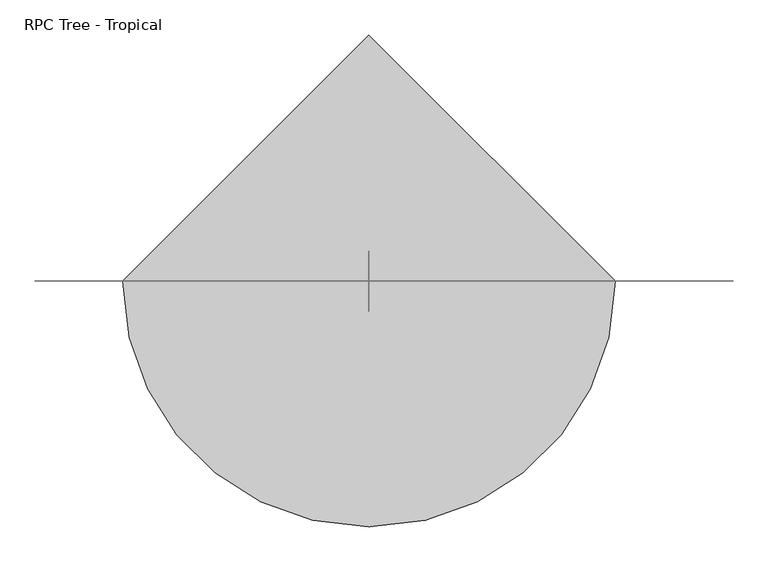
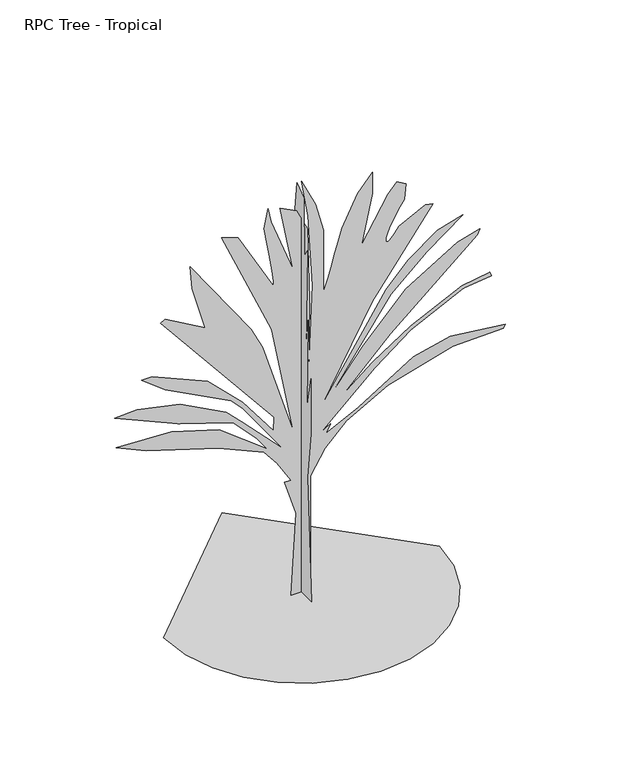
"""IFC4 building model written with IfcOpenShell, lengths in millimetres: geographic element geometry, RPC Tree - Tropical."""

from ifc_helpers import new_model, si_unit, origin, place, context, project, spatial, triangles, source, transform, mapped, element, save


def rpc_tree_tropical_0177ab4a(model_context):
    return source(origin(), model_context, "Body", "Tessellation", [
        triangles([(-93.7534889, -0.0079219, 0.0614497), (-47.9158571, -0.0079683, 779.2394274), (-154.8704887, -0.0079884, 1115.3806829), (-93.7534889, -0.0079881, 1110.2879705), (-221.0799467, -0.0080005, 1319.1040764), (-343.3142189, -0.0080096, 1471.8953316), (-755.8511021, -0.0080203, 1650.1526196), (-1417.9506592, -0.0080327, 1858.9686527), (-1692.9744244, -0.0080403, 1986.2938751), (-1183.6685932, -0.0080388, 1960.827697), (-750.7583897, -0.0080309, 1828.4099075), (-312.7554374, -0.0080109, 1492.2660358), (-409.5244217, -0.008019, 1629.7791538), (-623.4331673, -0.0080324, 1853.8733242), (-1122.5511028, -0.0080421, 2016.8526203), (-1708.2550323, -0.0080576, 2276.5982483), (-1499.4389992, -0.0080582, 2286.7861439), (-1107.2729656, -0.008053, 2200.2026207), (-689.6408993, -0.0080397, 1976.1084503), (-547.0350326, -0.0080312, 1833.5026199), (-170.149607, -0.0080081, 1446.4291534), (-531.7569317, -0.0080385, 1955.7349846), (-643.8040169, -0.0080455, 2072.8773983), (-1244.7860836, -0.0080643, 2388.6453335), (-1458.6948292, -0.0080743, 2556.7145805), (-1361.9258812, -0.0080743, 2556.7145805), (-857.7127625, -0.0080609, 2332.6230263), (-536.8496078, -0.0080424, 2021.9453327), (-256.7306412, -0.00802, 1645.0599072), (-251.6384557, -0.0080279, 1777.4776966), (-1285.5302536, -0.0081034, 3045.6393883), (-1244.7860836, -0.008105, 3071.1157402), (-878.0860828, -0.0080922, 2857.1968208), (-1000.3185928, -0.0081174, 3279.9291573), (-1015.5992735, -0.0081302, 3493.8480766), (-460.4539802, -0.0080828, 2699.3102371), (-353.4996074, -0.00807, 2485.4142815), (-73.3816582, -0.0080157, 1573.756992), (-272.0112855, -0.0080789, 2633.1177658), (-730.3875401, -0.0081411, 3677.1854324), (-577.5937778, -0.0081377, 3621.1783859), (-261.8258789, -0.0081041, 3055.8248131), (-253.7766246, -0.0081039, 3053.36101), (-254.8154783, -0.0081061, 3089.6323425), (-263.4286335, -0.0081101, 3158.2124588), (-278.0996675, -0.0081158, 3252.5988487), (-297.3122485, -0.0081226, 3366.3907402), (-319.5550223, -0.0081301, 3493.0862045), (-343.3142189, -0.008138, 3626.2583084), (-302.5700489, -0.0081487, 3804.5157417), (-277.1039979, -0.0081408, 3672.1055099), (-78.4743615, -0.0081092, 3142.4134232), (-195.6149131, -0.0081469, 3773.9594673), (-42.8231537, -0.0081423, 3697.556282), (53.9453128, -0.0081299, 3488.742865), (74.3173933, -0.0080886, 2796.084272), (64.1312281, -0.008043, 2032.1306122), (99.7824359, -0.0080965, 2928.5200836), (59.0382705, -0.0081371, 3610.9929611), (3.0145246, -0.0081581, 3962.4023254), (130.3409359, -0.0081423, 3697.556282), (201.643851, -0.0081259, 3422.5503937), (201.643851, -0.008091, 2836.8259712), (206.54377, -0.0080912, 2840.5597549), (220.2640989, -0.0080935, 2878.5074387), (241.3341791, -0.0080974, 2944.9539642), (268.285114, -0.0081028, 3034.2095627), (299.6439739, -0.0081091, 3140.5594666), (333.9441513, -0.0081161, 3258.339196), (369.7149693, -0.0081235, 3381.7834053), (512.3208361, -0.0081405, 3667.0000076), (649.833954, -0.0081499, 3824.8865913), (649.833954, -0.0081377, 3621.1783859), (547.9722937, -0.0081101, 3157.7043503), (792.4397844, -0.0081341, 3560.0405479), (873.9281244, -0.0081399, 3656.8145828), (955.4164644, -0.0081368, 3605.8877495), (940.1383272, -0.0081283, 3463.2918022), (902.2287952, -0.0081247, 3401.3412231), (866.0592007, -0.008121, 3341.0669952), (833.3617779, -0.0081176, 3284.0693115), (805.8763916, -0.0081145, 3232.0248138), (785.3405085, -0.0081119, 3186.5842735), (773.4913771, -0.0081096, 3149.3731728), (772.066464, -0.008108, 3122.0428642), (778.9574678, -0.0081071, 3107.4885201), (790.3900549, -0.008107, 3106.0406433), (805.6096928, -0.0081076, 3115.4894852), (823.8595963, -0.0081087, 3133.6758751), (844.3802914, -0.0081102, 3158.4156441), (866.4147749, -0.0081119, 3187.5240417), (889.2062616, -0.0081138, 3218.8168991), (1133.6737524, -0.008121, 3341.0417061), (1199.8839552, -0.0081201, 3325.7763588), (649.833954, -0.0080755, 2577.0854301), (171.0856145, -0.0080239, 1711.2701099), (772.066464, -0.0080798, 2648.3834038), (975.7897848, -0.0080925, 2862.3023232), (1240.6281979, -0.0081041, 3055.8248131), (1474.9102638, -0.0081083, 3127.1480759), (1148.9544331, -0.0080937, 2882.6728821), (817.9058899, -0.0080761, 2587.2708549), (247.4814783, -0.0080279, 1777.4776966), (568.3456504, -0.0080521, 2184.9244835), (950.323752, -0.0080764, 2592.3763573), (1423.9781982, -0.0080934, 2877.5676704), (1632.7942314, -0.0080968, 2933.6000061), (1607.3281986, -0.008094, 2887.7783844), (812.810634, -0.0080537, 2210.3880455), (369.7149693, -0.0080272, 1767.2924171), (649.833954, -0.0080406, 1991.3865875), (1001.2558903, -0.0080543, 2220.5759411), (1464.7223682, -0.0080676, 2444.6699661), (1724.470467, -0.00807, 2485.4142815), (1734.6558918, -0.0080676, 2444.6699661), (1480.0029762, -0.0080658, 2414.1113663), (1001.2558903, -0.0080518, 2179.8317711), (670.2048037, -0.008037, 1930.2715679), (181.271766, -0.0080099, 1476.9878986), (267.853309, -0.0080133, 1533.012822), (227.1093933, -0.0080084, 1451.5218658), (522.5062245, -0.0080172, 1599.2204086), (1021.6266672, -0.0080361, 1914.9909599), (1362.8631786, -0.0080406, 1991.3865875), (1861.983585, -0.0080373, 1935.3642803), (1846.702977, -0.0080351, 1899.7128227), (1383.2340282, -0.0080345, 1889.5247818), (792.4397844, -0.0080242, 1716.3628223), (410.4591393, -0.0080118, 1507.5467892), (216.9232418, -0.0080002, 1314.0087479), (84.5035629, -0.0079872, 1095.0072899), (84.5035629, -0.0079219, 0.0), (0.0460873, 53.9902683, 0.0519176), (0.0460761, -156.8964007, 0.0519049), (0.0460873, -97.584823, 1166.5210207), (0.0460761, -150.306614, 1621.2474072), (0.0460761, -150.3063596, 2148.4652264), (0.0460873, -90.9945366, 1832.1335175), (0.0460873, -104.1746006, 2688.8710487), (0.0460873, -71.2236731, 2379.1228043), (0.0460873, -97.584823, 3354.4783859), (0.0460873, -51.4530639, 3275.3826324), (0.0460873, -44.8630274, 3828.9758766), (0.0460982, 67.1710998, 3908.0460503), (0.0460982, 133.0732182, 3374.239389), (0.0460982, 152.8438319, 2609.7752953), (0.0460982, 106.7123182, 1950.7591255), (0.0460873, 53.9902683, 1120.3895342), (-1259.0684967, 0.0, 0.0575648), (-1225.7818657, -288.495908, 0.0575478), (-1130.983873, -553.4307541, 0.0575321), (-982.2667877, -787.2201176, 0.0575181), (-787.2201176, -982.2667877, 0.0575064), (-553.4307541, -1130.983873, 0.0574975), (-288.495908, -1225.7818657, 0.0574919), (4.41e-05, -1259.0684967, 0.0574899), (288.495908, -1225.7818657, 0.0574919), (553.4307541, -1130.983873, 0.0574975), (787.2201176, -982.2667877, 0.0575064), (982.2667877, -787.2201176, 0.0575181), (1130.983873, -553.4307541, 0.0575321), (1225.7818657, -288.495908, 0.0575478), (1259.0684967, 0.0001101, 0.0575648), (-0.0001766, 1259.0684967, 0.05764)], [[59, 60, 61], [99, 100, 101], [8, 9, 10], [49, 50, 51], [98, 99, 101], [15, 16, 17], [15, 17, 18], [119, 120, 121], [34, 35, 36], [33, 34, 36], [98, 101, 102], [97, 98, 102], [24, 25, 26], [24, 26, 27], [23, 24, 27], [23, 27, 28], [22, 23, 28], [22, 28, 29], [21, 22, 29], [7, 8, 10], [7, 10, 11], [71, 72, 73], [106, 107, 108], [106, 108, 109], [105, 106, 109], [104, 105, 109], [104, 109, 110], [103, 104, 110], [39, 40, 41], [39, 41, 42], [52, 53, 54], [52, 54, 55], [52, 55, 56], [59, 61, 62], [58, 59, 62], [58, 62, 63], [57, 58, 63], [7, 11, 12], [6, 7, 12], [15, 18, 19], [14, 15, 19], [14, 19, 20], [13, 14, 20], [13, 20, 21], [12, 13, 21], [93, 94, 95], [92, 93, 95], [91, 92, 95], [90, 91, 95], [89, 90, 95], [88, 89, 95], [87, 88, 95], [2, 3, 4], [96, 97, 102], [96, 102, 103], [124, 125, 126], [124, 126, 127], [39, 42, 43], [49, 51, 52], [48, 49, 52], [47, 48, 52], [46, 47, 52], [45, 46, 52], [44, 45, 52], [86, 87, 95], [114, 115, 116], [113, 114, 116], [30, 31, 32], [30, 32, 33], [30, 33, 36], [30, 36, 37], [30, 37, 38], [29, 30, 38], [21, 29, 38], [131, 132, 1], [131, 1, 2], [131, 2, 4], [5, 6, 12], [5, 12, 21], [123, 124, 127], [123, 127, 128], [122, 123, 128], [122, 128, 129], [121, 122, 129], [121, 129, 130], [113, 116, 117], [112, 113, 117], [111, 112, 117], [111, 117, 118], [110, 111, 118], [110, 118, 119], [103, 110, 119], [96, 103, 119], [71, 73, 74], [70, 71, 74], [69, 70, 74], [68, 69, 74], [44, 52, 56], [43, 44, 56], [39, 43, 56], [39, 56, 57], [38, 39, 57], [75, 76, 77], [75, 77, 78], [74, 75, 78], [74, 78, 79], [74, 79, 80], [74, 80, 81], [74, 81, 82], [74, 82, 83], [74, 83, 84], [74, 84, 85], [67, 68, 74], [119, 121, 130], [130, 131, 4], [130, 4, 5], [130, 5, 21], [119, 130, 21], [119, 21, 38], [96, 119, 38], [96, 38, 57], [95, 96, 57], [95, 57, 63], [95, 63, 64], [86, 95, 64], [86, 64, 65], [86, 65, 66], [86, 66, 67], [86, 67, 74], [86, 74, 85], [138, 139, 140], [136, 137, 138], [140, 141, 142], [143, 144, 145], [142, 143, 145], [142, 145, 146], [140, 142, 146], [140, 146, 147], [138, 140, 147], [138, 147, 148], [136, 138, 148], [135, 136, 148], [134, 135, 148], [134, 148, 133], [163, 164, 149], [162, 163, 149], [162, 149, 150], [161, 162, 150], [161, 150, 151], [161, 151, 152], [160, 161, 152], [159, 160, 152], [159, 152, 153], [159, 153, 154], [159, 154, 155], [159, 155, 156], [159, 156, 157], [159, 157, 158]], closed=False),
    ])


if __name__ == "__main__":
    model = new_model("IFC4")
    model_context = context("Model", 3, world=origin())
    ifc_project = project(units=[si_unit("LENGTHUNIT", "METRE", prefix="MILLI")], contexts=[model_context])
    site = spatial("IfcSite", under=ifc_project)
    building = spatial("IfcBuilding", under=site)
    placement = place(None, origin())
    rpc_tree_tropical_shape = rpc_tree_tropical_0177ab4a(model_context)
    element("IfcGeographicElement", 1, ObjectType="RPC Tree - Tropical", at=placement, inside=building, context=model_context, shape_type="MappedRepresentation", body=[
        mapped(rpc_tree_tropical_shape, transform((0.0, 0.0, 0.0), x_axis=(1.0, 0.0, 0.0), y_axis=(0.0, 1.0, 0.0), z_axis=(0.0, 0.0, 1.0))),
    ])
    save(model, "model.ifc")

# Revit data of these elements
# Type "RPC Tree - Tropical"
#   built-in parameter 1005198 = "{2, 15},{39, RPC-16-G2M6-EAFX-C5H6-W000-ST1L-LVER-AU},{1, 0},{1, 0},{2, 13},{1, 8},{5, Color},{1, 0},{1, 0},{3, 0.8},{3, 0.8},{3, 0.8},{1, 8},{7, BBoxMin},{1, 0},{1, 0},{1, 0},{1, 0},{1, 0},{1, 8},{7, BBoxMax},{1, 0},{1, 0},{1, 0},{1, 0},{1, 0},{2, 11},{9, RPCTypeId},{1, 0},{1, 0},{39, RPC-16-G2M6-EAFX-C5H6-W000-ST1L-LVER-AU},{1, 6},{14, RPCPlantHeight},{1, 0},{1, 0},{2, 13},{2, 11},{7, keyword},{1, 0},{1, 0},{35, :RPCs:Trees [Tropical]:Geometry:RPC},{2, 11},{8, category},{1, 0},{1, 0},{16, Trees [Tropical]},{2, 11},{12, LocalizedUID},{1, 0},{1, 0},{15, Traveler's Palm},{2, 14},{6, Height},{1, 0},{1, 0},{2, 13},{1, 2},{16, Cast Reflections},{1, 0},{1, 0},{1, 0},{1, 2},{12, Cast Shadows},{1, 0},{1, 0},{1, 1},{1, 2},{9, Lock View},{1, 0},{1, 0},{1, 0},{1, 4},{5, ViewC},{1, 0},{1, 0},{1, 0},{21, assetlibrary_base.fbx},{1, 5},"
#   built-in parameter 1005195 = "RPC-16-G2M6-EAFX-C5H6-W000-ST1L-LVER-AU"
#   Assembly Code = "G2050500"
#   Height = 13' - 0"
#   Plan Symbol = element 321958
#   Default Elevation = 0
